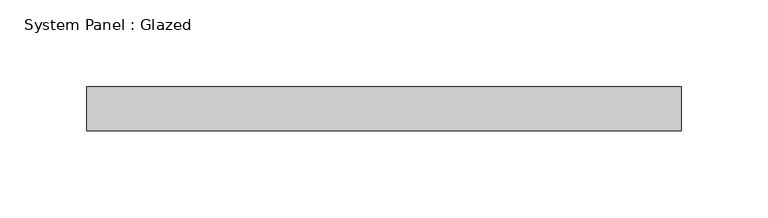
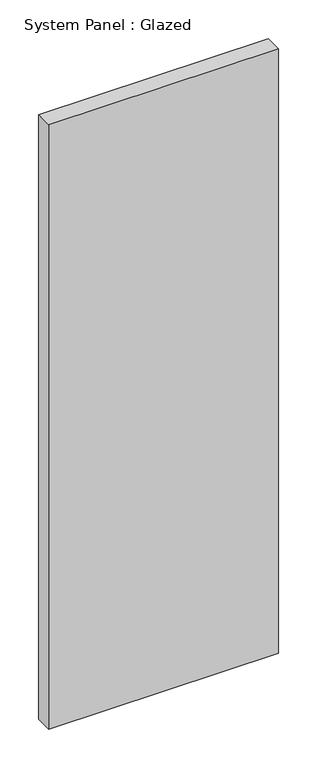
"""IFC4 building model written with IfcOpenShell, lengths in millimetres: plate geometry, System Panel : Glazed."""

from ifc_helpers import new_model, si_unit, origin, origin_with_axes, place, context, project, spatial, polyline, outline, extrude, source, transform, mapped, element, save


def system_panel_glazed_809156e5(model_context):
    return source(origin(), model_context, "Body", "SweptSolid", [
        extrude(outline(polyline([(171.45, 19.05), (-171.45, 19.05), (-171.45, 44.45), (171.45, 44.45), (171.45, 19.05)])), origin_with_axes(), (0.0, 0.0, 1.0), 952.5),
    ])


if __name__ == "__main__":
    model = new_model("IFC4")
    model_context = context("Model", 3, world=origin())
    ifc_project = project(units=[si_unit("LENGTHUNIT", "METRE", prefix="MILLI")], contexts=[model_context])
    site = spatial("IfcSite", under=ifc_project)
    building = spatial("IfcBuilding", under=site)
    placement = place(None, origin())
    system_panel_glazed_shape = system_panel_glazed_809156e5(model_context)
    element("IfcPlate", 1, ObjectType="System Panel : Glazed", at=placement, inside=building, context=model_context, shape_type="MappedRepresentation", body=[
        mapped(system_panel_glazed_shape, transform((0.0, 0.0, 0.0), x_axis=(1.0, 0.0, 0.0), y_axis=(0.0, 1.0, 0.0), z_axis=(0.0, 0.0, 1.0))),
    ])
    save(model, "model.ifc")

# Revit data of these elements
# Type "System Panel : Glazed"
#   Construction Type Id = "GSP4R"
#   Analytic Construction = "1/8 in Pilkington single glazing"
#   Visual Light Transmittance = 0.9
#   Solar Heat Gain Coefficient = 0.86
#   Heat Transfer Coefficient (U) = 1.18115 BTU/(h·ft²·°F)
#   Define Thermal Properties by = 1
# Element 1 (IfcPlate, "System Panel : Glazed")
#   Materials on its faces: "Glass"
# Materials
#   "Glass": class "Glass", colour RGB 0 128 192, transparency 0.75, Description = "Soda Lime Glass", Cost = 0
